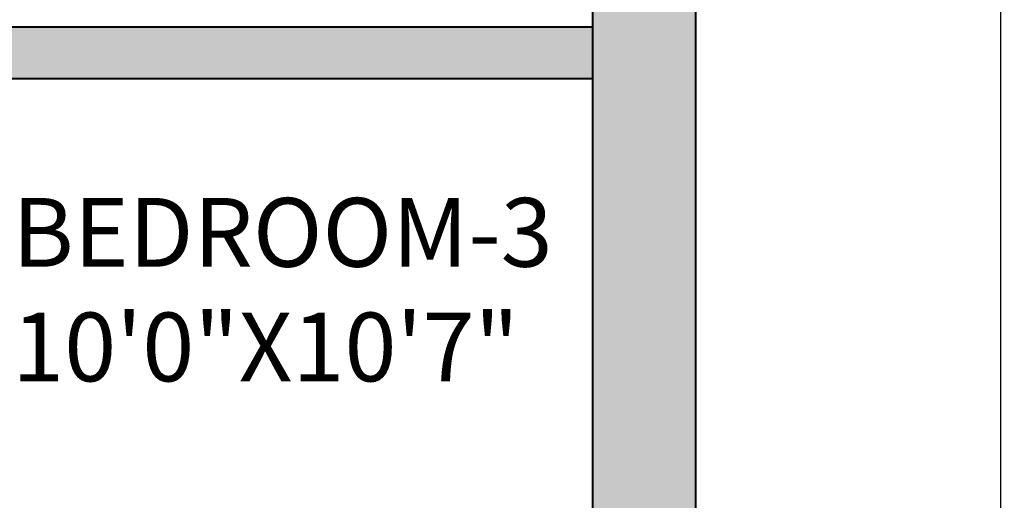
# Model space of a CAD drawing. Units: inches. Extents: x 1441 to 2460, y 1648 to 2683.
# Tile 10 of 35: x 1830 to 1916, y 1933 to 1975. Entities that reach past the tile are written whole.
import ezdxf

# ---------------------------------------------------------------- set-up
doc = ezdxf.new("R2010")
doc.units = ezdxf.units.IN
for name, color, linetype, lineweight in [('A-ANNO-DIMS', 2, 'Continuous', 18), ('A-AREA-IDEN', 7, 'Continuous', 20), ('A-WALL', 7, 'Continuous', 40)]:
    doc.layers.add(name, color=color, linetype=linetype, lineweight=lineweight)
doc.layers.add('A-WALL-PATT', color=251, linetype='Continuous', lineweight=13, true_color=0x636466)
doc.styles.get("Standard").update_dxf_attribs({"font": 'arial.ttf'})
doc.dimstyles.get("Standard").update_dxf_attribs({"dimtxt": 0.18, "dimasz": 0.18, "dimexe": 0.18, "dimexo": 0.0625, "dimgap": 0.09, "dimtad": 0, "dimtih": 1, "dimtoh": 1, "dimdec": 4, "dimzin": 0, "dimdsep": 46, "dimtxsty": 'Standard', "dimcen": 0.09, "dimadec": 0, "dimazin": 0, "dimtfac": 1, "dimtdec": 4, "dimtofl": 0, "dimtmove": 0, "dimatfit": 3, "dimfxl": 1, "dimtolj": 1, "dimtzin": 0, "dimarcsym": 0})

# ---------------------------------------------------------------- blocks, each defined once
blk = doc.blocks.new('*D67')
at = {"layer": 'A-ANNO-DIMS', "color": 0, "lineweight": -2, "transparency": 16777216}
for p, q in [((1889.448, 2298.695), (1916.216, 2298.695)), ((1916.036, 2298.515), (1916.036, 2055.938)), ((1916.036, 1812.997), (1916.036, 2055.574)), ((1758.224, 1812.817), (1916.216, 1812.817))]:
    blk.add_line(p, q, dxfattribs=at)
at = {"layer": 'A-ANNO-DIMS', "color": 0, "transparency": 16777216}
for points in [[(1916.006, 2298.515), (1916.066, 2298.515), (1916.036, 2298.695)], [(1916.006, 1812.997), (1916.066, 1812.997), (1916.036, 1812.817)]]:
    blk.add_solid(points, dxfattribs=at)
at = {"layer": 'Defpoints', "color": 0, "transparency": 16777216}
for p in [(1889.386, 2298.695), (1916.036, 2298.695), (1758.161, 1812.817)]:
    blk.add_point(p, dxfattribs=at)
at = {"layer": 'A-ANNO-DIMS', "color": 0, "transparency": 16777216, "insert": (1916.036, 2055.756), "char_height": 0.18, "attachment_point": 5}
blk.add_mtext('\\A1;485.9', dxfattribs=at)

msp = doc.modelspace()

# ---------------------------------------------------------------- hatches: boundary and pattern name
at = {"layer": 'A-WALL-PATT'}
h = msp.add_hatch(color=256, dxfattribs=at)
h.dxf.hatch_style = 1
h.paths.add_polyline_path([(1627.5085, 2298.6952), (1568.8859, 2298.6952), (1568.8859, 2246.9605), (1577.8859, 2246.9605), (1577.8859, 2289.6952), (1627.5085, 2289.6952), (1627.5085, 2294.1952)])
h.paths.add_polyline_path([(1675.5777, 2298.6952), (1651.5085, 2298.6952), (1651.5085, 2289.6952), (1675.5777, 2289.6952), (1675.5777, 2294.1952)])
h.paths.add_polyline_path([(1667.3859, 2289.6952), (1662.8859, 2289.6952), (1662.8859, 2233.0622), (1667.3859, 2233.0622)])
h.paths.add_polyline_path([(1715.8721, 2294.3362), (1715.8721, 2295.2788), (1715.8721, 2298.6952), (1699.5777, 2298.6952), (1699.5777, 2289.6952), (1715.8721, 2289.6952)])
h.paths.add_polyline_path([(1707.8859, 2289.6952), (1703.3859, 2289.6952), (1703.3859, 2199.6952), (1707.8859, 2199.6952)])
h.paths.add_polyline_path([(1760.3859, 2204.637), (1755.8859, 2204.637), (1755.8859, 2199.6952), (1667.3859, 2199.6952), (1667.3859, 2204.637), (1662.8859, 2204.637), (1662.8859, 2195.1952), (1760.3859, 2195.1952)])
h.paths.add_polyline_path([(1760.3859, 2289.6952), (1755.8859, 2289.6952), (1755.8859, 2233.0622), (1760.3859, 2233.0622)])
h.paths.add_polyline_path([(1889.3859, 2298.6952), (1739.8721, 2298.6952), (1739.8721, 2289.6952), (1880.3859, 2289.6952), (1880.3859, 2250.8051), (1889.3859, 2250.8051)])
h.paths.add_polyline_path([(1889.3859, 2202.8051), (1880.3859, 2202.8051), (1880.3859, 2157.6952), (1747.948, 2157.6952), (1747.948, 2153.1952), (1755.8859, 2153.1952), (1755.8859, 2058.005), (1760.3859, 2058.005), (1760.3859, 2153.1952), (1880.3859, 2153.1952), (1880.3859, 2124.108), (1889.3859, 2124.108)])
h.paths.add_polyline_path([(1889.3859, 1984.8305), (1880.3859, 1984.8305), (1880.3859, 1834.1952), (1889.3859, 1834.1952)])
h.paths.add_polyline_path([(1889.3859, 2076.108), (1880.3859, 2076.108), (1880.3859, 2008.8305), (1889.3859, 2008.8305)])
h.paths.add_polyline_path([(1880.3859, 2027.1952), (1800.8859, 2027.1952), (1800.8859, 2000.9452), (1805.3859, 2000.9452), (1805.3859, 2022.6952), (1880.3859, 2022.6952)])
h.paths.add_polyline_path([(1800.8859, 2027.1952), (1760.3859, 2027.1952), (1760.3859, 2030.7912), (1755.8859, 2030.7912), (1755.8859, 2022.6952), (1800.8859, 2022.6952)])
h.paths.add_polyline_path([(1880.3859, 1974.6952), (1805.3859, 1974.6952), (1805.3859, 1978.7973), (1800.8859, 1978.7973), (1800.8859, 1974.6952), (1794.8823, 1974.6952), (1794.8823, 1970.1952), (1800.8859, 1970.1952), (1805.3859, 1970.1952), (1880.3859, 1970.1952)])
h.paths.add_polyline_path([(1760.3859, 1974.6952), (1755.8859, 1974.6952), (1755.8859, 1925.6952), (1751.8616, 1925.6952), (1751.8616, 1921.1952), (1760.3859, 1921.1952)])
h.paths.add_polyline_path([(1760.3859, 1921.1952), (1755.8859, 1921.1952), (1755.8859, 1843.1952), (1760.3859, 1843.1952)])
h.paths.add_polyline_path([(1799.1136, 1838.6952), (1799.1136, 1843.1952), (1760.3859, 1843.1952), (1751.8944, 1843.1952), (1751.8944, 1834.1952), (1758.1615, 1834.1952), (1799.1136, 1834.1952)])
h.paths.add_polyline_path([(1880.3859, 1843.1952), (1859.1136, 1843.1952), (1859.1136, 1834.1952), (1880.3859, 1834.1952)])
h.paths.add_polyline_path([(1577.8859, 1857.7914), (1568.8859, 1857.7914), (1568.8859, 1834.1952), (1695.0034, 1834.1952), (1695.0034, 1838.6952), (1695.0034, 1843.1952), (1577.8859, 1843.1952)])
h.paths.add_polyline_path([(1577.8859, 1959.2399), (1573.3859, 1959.2399), (1568.8859, 1959.2399), (1568.8859, 1905.7914), (1577.8859, 1905.7914), (1577.8859, 1921.1952), (1703.3859, 1921.1952), (1707.8859, 1921.1952), (1715.1501, 1921.1952), (1715.1501, 1925.6952), (1707.8859, 1925.6952), (1703.3859, 1925.6952), (1577.8859, 1925.6952)])
h.paths.add_polyline_path([(1577.8859, 2106.6907), (1568.8859, 2106.6907), (1568.8859, 2019.2399), (1577.8859, 2019.2399)])
h.paths.add_polyline_path([(1707.8859, 2051.6952), (1703.3859, 2051.6952), (1703.3859, 2048.6952), (1703.3859, 1925.6952), (1707.8859, 1925.6952)])
h.paths.add_polyline_path([(1703.3859, 2051.6952), (1676.3859, 2051.6952), (1676.3859, 2048.6952), (1703.3859, 2048.6952)])
h.paths.add_polyline_path([(1703.3859, 2102.6952), (1676.3859, 2102.6952), (1676.3859, 2099.6952), (1685.3859, 2099.6952), (1703.3859, 2099.6952)])
h.paths.add_polyline_path([(1707.8859, 2153.1952), (1710.5611, 2153.1952), (1710.5611, 2157.6952), (1707.8859, 2157.6952), (1707.8859, 2195.1952), (1703.3859, 2195.1952), (1703.3859, 2099.6952), (1707.8859, 2099.6952)])
h.paths.add_polyline_path([(1577.8859, 2198.9605), (1568.8859, 2198.9605), (1568.8859, 2166.6907), (1577.8859, 2166.6907)])

# ---------------------------------------------------------------- linework, layer by layer
at = {"layer": 'A-WALL'}
for p, q in [((1889.3859, 2298.6952), (1889.3859, 1834.1952)), ((1880.3859, 2153.1952), (1880.3859, 1834.1952)), ((1805.3859, 1974.6952), (1880.3859, 1974.6952)), ((1800.8859, 1970.1952), (1880.3859, 1970.1952))]:
    msp.add_line(p, q, dxfattribs=at)

# ---------------------------------------------------------------- texts
at = {"layer": 'A-AREA-IDEN', "insert": (1829.7048, 1959.7547), "char_height": 6, "attachment_point": 1}
msp.add_mtext_dynamic_manual_height_columns('BEDROOM-3\\P10\'0"X10\'7"', width=85.554017, gutter_width=12.5, heights=[0], dxfattribs=at)

# ---------------------------------------------------------------- dimensions: what is measured, and where the dimension line sits
at = {"layer": 'A-ANNO-DIMS'}
dim = msp.add_linear_dim(base=(1916.0359, 2298.6952), p1=(1758.1615, 1812.8171), p2=(1889.3859, 2298.6952), angle=90, dimstyle='Standard', override={"dimdec": 1, "dimlfac": 1, "dimrnd": 0, "dimzin": 0, "dimdsep": 46, "dimlunit": 2}, dxfattribs=at)
dim.commit()
dim.dimension.update_dxf_attribs({"geometry": '*D67', "text_midpoint": (1916.0359, 2055.7561)})

doc.saveas('drawing.dxf')
